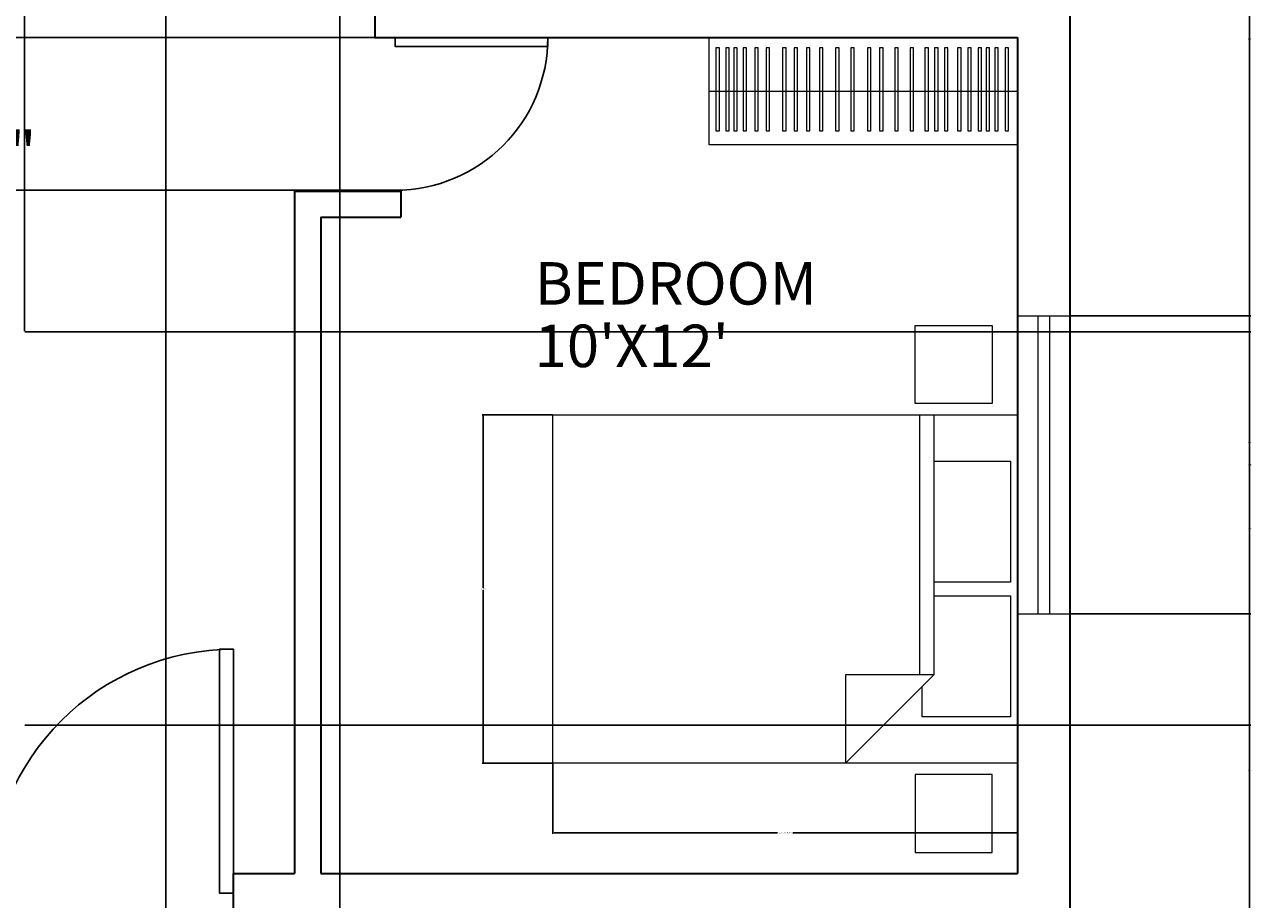
# Model space of a CAD drawing. Units: inches. Extents: x 25018 to 25490, y 41421 to 42101.
# Tile 4 of 5: x 25279 to 25490, y 41707 to 41858. Entities that reach past the tile are written whole.
import ezdxf

# ---------------------------------------------------------------- set-up
doc = ezdxf.new("R2010")
doc.units = ezdxf.units.IN
for name, color, linetype, lineweight in [('A-ANNO-DIMS', 2, 'Continuous', 18), ('A-AREA-IDEN', 7, 'Continuous', 18), ('A-DOOR', 3, 'Continuous', 25), ('A-FURN', 8, 'Continuous', 18), ('A-GLAZ', 4, 'Continuous', 18), ('A-WALL', 7, 'Continuous', 35)]:
    doc.layers.add(name, color=color, linetype=linetype, lineweight=lineweight)
doc.styles.get("Standard").update_dxf_attribs({"font": 'arial.ttf'})
doc.dimstyles.get("Standard").update_dxf_attribs({"dimtxt": 0.18, "dimasz": 0.18, "dimexe": 0.18, "dimexo": 0.0625, "dimgap": 0.09, "dimtad": 0, "dimtih": 1, "dimtoh": 1, "dimdec": 4, "dimzin": 0, "dimdsep": 46, "dimtxsty": 'Standard', "dimcen": 0.09, "dimadec": 0, "dimazin": 0, "dimtfac": 1, "dimtdec": 4, "dimtofl": 0, "dimtmove": 0, "dimatfit": 3, "dimfxl": 1, "dimtolj": 1, "dimtzin": 0, "dimarcsym": 0})

# ---------------------------------------------------------------- blocks, each defined once
blk = doc.blocks.new('*U2')
for p, q in [((0, 0), (0, -100)), ((750, 0), (750, -100))]:
    blk.add_line(p, q)
blk.add_lwpolyline([(0, 0), (0, 750), (43.75, 750), (43.75, 0)], close=True)
blk.add_arc((0, 0), 750, 0, 90)
blk = doc.blocks.new('Bed - Queen')
for p, q in [((0, -80.00003), (0, 0)), ((0, 0), (59.99999, 0)), ((59.99999, 0), (59.99999, -80.00003)), ((7.99999, -1.2), (28.79998, -1.2)), ((7.99999, -14.4), (7.99999, -1.2)), ((28.79998, -1.2), (28.79998, -14.4)), ((31.19999, -1.2), (51.99999, -1.2)), ((31.19999, -14.4), (31.19999, -1.2)), ((51.99999, -1.2), (51.99999, -16.4)), ((0, -14.4), (44.8, -14.4)), ((59.99999, -29.6), (44.8, -14.4)), ((44.8, -14.4), (44.8, -29.6)), ((44.8, -16.8), (0, -16.8)), ((51.99999, -16.4), (46.79936, -16.4)), ((44.8, -29.6), (59.99999, -29.6)), ((59.99999, -80.00003), (0, -80.00003))]:
    blk.add_line(p, q)
blk = doc.blocks.new('WARDROBE-SLATTED')
blk.add_line((0, 9.22), (53.1, 9.22))
for points in [[(0, 0), (53.1, 0), (53.1, 18.45), (0, 18.45)], [(1.16, 16.06), (1.76, 16.06), (1.76, 1.75), (1.16, 1.75)], [(2.87, 16.06), (3.47, 16.06), (3.47, 1.75), (2.87, 1.75)], [(4.23, 16.06), (4.83, 16.06), (4.83, 1.75), (4.23, 1.75)], [(5.83, 16.06), (6.43, 16.06), (6.43, 1.75), (5.83, 1.75)], [(7.85, 16.06), (8.45, 16.06), (8.45, 1.75), (7.85, 1.75)], [(9.82, 16.06), (10.42, 16.06), (10.42, 1.75), (9.82, 1.75)], [(12.64, 16.06), (13.24, 16.06), (13.24, 1.75), (12.64, 1.75)], [(14.63, 16.06), (15.23, 16.06), (15.23, 1.75), (14.63, 1.75)], [(16.74, 16.06), (17.34, 16.06), (17.34, 1.75), (16.74, 1.75)], [(18.99, 16.06), (19.59, 16.06), (19.59, 1.75), (18.99, 1.75)], [(21.77, 16.06), (22.37, 16.06), (22.37, 1.75), (21.77, 1.75)], [(24.4, 16.06), (25, 16.06), (25, 1.75), (24.4, 1.75)], [(27.25, 16.06), (27.85, 16.06), (27.85, 1.75), (27.25, 1.75)], [(29.36, 16.06), (29.96, 16.06), (29.96, 1.75), (29.36, 1.75)], [(31.98, 16.06), (32.58, 16.06), (32.58, 1.75), (31.98, 1.75)], [(34.61, 16.06), (35.21, 16.06), (35.21, 1.75), (34.61, 1.75)], [(37.17, 16.06), (37.77, 16.06), (37.77, 1.75), (37.17, 1.75)], [(38.82, 16.06), (39.42, 16.06), (39.42, 1.75), (38.82, 1.75)], [(40.51, 16.06), (41.11, 16.06), (41.11, 1.75), (40.51, 1.75)], [(42.78, 16.06), (43.38, 16.06), (43.38, 1.75), (42.78, 1.75)], [(44.55, 16.06), (45.15, 16.06), (45.15, 1.75), (44.55, 1.75)], [(46.32, 16.06), (46.92, 16.06), (46.92, 1.75), (46.32, 1.75)], [(47.7, 16.06), (48.3, 16.06), (48.3, 1.75), (47.7, 1.75)], [(49.2, 16.06), (49.8, 16.06), (49.8, 1.75), (49.2, 1.75)], [(50.97, 16.06), (51.57, 16.06), (51.57, 1.75), (50.97, 1.75)]]:
    blk.add_lwpolyline(points, close=True)
blk = doc.blocks.new('TABLE-BEDSIDE')
blk.add_lwpolyline([(0, 13.4), (13.26, 13.4), (13.26, 0), (0, 0)], close=True)
blk = doc.blocks.new('*D18')
at = {"layer": 'A-ANNO-DIMS', "color": 0, "lineweight": -2, "transparency": 16777216}
for p, q in [((25369.65, 41730.48), (25369.65, 41718.36)), ((25449.65, 41730.48), (25449.65, 41718.36)), ((25369.83, 41718.54), (25408.35, 41718.54)), ((25449.47, 41718.54), (25410.96, 41718.54))]:
    blk.add_line(p, q, dxfattribs=at)
at = {"layer": 'A-ANNO-DIMS', "color": 0, "transparency": 16777216}
for points in [[(25369.83, 41718.57), (25369.83, 41718.51), (25369.65, 41718.54)], [(25449.47, 41718.57), (25449.47, 41718.51), (25449.65, 41718.54)]]:
    blk.add_solid(points, dxfattribs=at)
at = {"layer": 'Defpoints', "color": 0, "transparency": 16777216}
for p in [(25369.65, 41730.54), (25449.65, 41730.54), (25449.65, 41718.54)]:
    blk.add_point(p, dxfattribs=at)
at = {"layer": 'A-ANNO-DIMS', "color": 0, "transparency": 16777216, "insert": (25409.65, 41718.54), "char_height": 0.18, "attachment_point": 5}
blk.add_mtext('\\A1;QUEEN BED 80 TYP.', dxfattribs=at)
blk = doc.blocks.new('*D19')
at = {"layer": 'A-ANNO-DIMS', "color": 0, "lineweight": -2, "transparency": 16777216}
for p, q in [((25369.59, 41790.54), (25357.47, 41790.54)), ((25357.65, 41790.36), (25357.65, 41760.72)), ((25357.65, 41730.72), (25357.65, 41760.36)), ((25369.59, 41730.54), (25357.47, 41730.54))]:
    blk.add_line(p, q, dxfattribs=at)
at = {"layer": 'A-ANNO-DIMS', "color": 0, "transparency": 16777216}
for points in [[(25357.62, 41790.36), (25357.68, 41790.36), (25357.65, 41790.54)], [(25357.62, 41730.72), (25357.68, 41730.72), (25357.65, 41730.54)]]:
    blk.add_solid(points, dxfattribs=at)
at = {"layer": 'Defpoints', "color": 0, "transparency": 16777216}
for p in [(25369.65, 41790.54), (25357.65, 41730.54), (25369.65, 41730.54)]:
    blk.add_point(p, dxfattribs=at)
at = {"layer": 'A-ANNO-DIMS', "color": 0, "transparency": 16777216, "insert": (25357.65, 41760.54), "char_height": 0.18, "attachment_point": 5}
blk.add_mtext('\\A1;60 TYP.', dxfattribs=at)
blk = doc.blocks.new('*D39')
at = {"layer": 'A-ANNO-DIMS', "color": 0, "lineweight": -2, "transparency": 16777216}
for p, q in [((25458.72, 42070.05), (25489.83, 42070.05)), ((25489.65, 42069.87), (25489.65, 41785.98)), ((25489.65, 41501.73), (25489.65, 41785.62)), ((25458.72, 41501.55), (25489.83, 41501.55))]:
    blk.add_line(p, q, dxfattribs=at)
at = {"layer": 'A-ANNO-DIMS', "color": 0, "transparency": 16777216}
for points in [[(25489.62, 42069.87), (25489.68, 42069.87), (25489.65, 42070.05)], [(25489.62, 41501.73), (25489.68, 41501.73), (25489.65, 41501.55)]]:
    blk.add_solid(points, dxfattribs=at)
at = {"layer": 'Defpoints', "color": 0, "transparency": 16777216}
for p in [(25458.65, 42070.05), (25489.65, 42070.05), (25458.65, 41501.55)]:
    blk.add_point(p, dxfattribs=at)
at = {"layer": 'A-ANNO-DIMS', "color": 0, "transparency": 16777216, "insert": (25489.65, 41785.8), "char_height": 0.18, "attachment_point": 5}
blk.add_mtext('\\A1;568.5', dxfattribs=at)
blk = doc.blocks.new('*D54')
at = {"layer": 'A-ANNO-DIMS', "color": 0, "lineweight": -2, "transparency": 16777216}
for p, q in [((25458.72, 41756.26), (25489.83, 41756.26)), ((25489.65, 41756.08), (25489.65, 41729.59)), ((25489.65, 41702.73), (25489.65, 41729.22)), ((25458.72, 41702.55), (25489.83, 41702.55))]:
    blk.add_line(p, q, dxfattribs=at)
at = {"layer": 'A-ANNO-DIMS', "color": 0, "transparency": 16777216}
for points in [[(25489.62, 41756.08), (25489.68, 41756.08), (25489.65, 41756.26)], [(25489.62, 41702.73), (25489.68, 41702.73), (25489.65, 41702.55)]]:
    blk.add_solid(points, dxfattribs=at)
at = {"layer": 'Defpoints', "color": 0, "transparency": 16777216}
for p in [(25458.65, 41756.26), (25489.65, 41756.26), (25458.65, 41702.55)]:
    blk.add_point(p, dxfattribs=at)
at = {"layer": 'A-ANNO-DIMS', "color": 0, "transparency": 16777216, "insert": (25489.65, 41729.4), "char_height": 0.18, "attachment_point": 5}
blk.add_mtext('\\A1;53.71', dxfattribs=at)
blk = doc.blocks.new('*D55')
at = {"layer": 'A-ANNO-DIMS', "color": 0, "lineweight": -2, "transparency": 16777216}
for p, q in [((25458.72, 41807.63), (25489.83, 41807.63)), ((25489.65, 41807.45), (25489.65, 41782.13)), ((25489.65, 41756.44), (25489.65, 41781.76)), ((25458.72, 41756.26), (25489.83, 41756.26))]:
    blk.add_line(p, q, dxfattribs=at)
at = {"layer": 'A-ANNO-DIMS', "color": 0, "transparency": 16777216}
for points in [[(25489.62, 41807.45), (25489.68, 41807.45), (25489.65, 41807.63)], [(25489.62, 41756.44), (25489.68, 41756.44), (25489.65, 41756.26)]]:
    blk.add_solid(points, dxfattribs=at)
at = {"layer": 'Defpoints', "color": 0, "transparency": 16777216}
for p in [(25458.65, 41807.63), (25489.65, 41807.63), (25458.65, 41756.26)]:
    blk.add_point(p, dxfattribs=at)
at = {"layer": 'A-ANNO-DIMS', "color": 0, "transparency": 16777216, "insert": (25489.65, 41781.95), "char_height": 0.18, "attachment_point": 5}
blk.add_mtext('\\A1;51.38', dxfattribs=at)
blk = doc.blocks.new('*D56')
at = {"layer": 'A-ANNO-DIMS', "color": 0, "lineweight": -2, "transparency": 16777216}
for p, q in [((25458.72, 41903), (25489.83, 41903)), ((25489.65, 41902.82), (25489.65, 41855.5)), ((25489.65, 41807.81), (25489.65, 41855.13)), ((25458.72, 41807.63), (25489.83, 41807.63))]:
    blk.add_line(p, q, dxfattribs=at)
at = {"layer": 'A-ANNO-DIMS', "color": 0, "transparency": 16777216}
for points in [[(25489.62, 41902.82), (25489.68, 41902.82), (25489.65, 41903)], [(25489.62, 41807.81), (25489.68, 41807.81), (25489.65, 41807.63)]]:
    blk.add_solid(points, dxfattribs=at)
at = {"layer": 'Defpoints', "color": 0, "transparency": 16777216}
for p in [(25458.65, 41903), (25489.65, 41903), (25458.65, 41807.63)]:
    blk.add_point(p, dxfattribs=at)
at = {"layer": 'A-ANNO-DIMS', "color": 0, "transparency": 16777216, "insert": (25489.65, 41855.31), "char_height": 0.18, "attachment_point": 5}
blk.add_mtext('\\A1;95.36', dxfattribs=at)
blk = doc.blocks.new('*D70')
at = {"layer": 'A-ANNO-DIMS', "color": 0, "lineweight": -2, "transparency": 16777216}
for p, q in [((25250.45, 41903.49), (25250.45, 41420.7)), ((25302.95, 41903.49), (25302.95, 41420.7)), ((25250.63, 41420.88), (25276.38, 41420.88)), ((25302.77, 41420.88), (25277.03, 41420.88))]:
    blk.add_line(p, q, dxfattribs=at)
at = {"layer": 'A-ANNO-DIMS', "color": 0, "transparency": 16777216}
for points in [[(25250.63, 41420.91), (25250.63, 41420.85), (25250.45, 41420.88)], [(25302.77, 41420.91), (25302.77, 41420.85), (25302.95, 41420.88)]]:
    blk.add_solid(points, dxfattribs=at)
at = {"layer": 'Defpoints', "color": 0, "transparency": 16777216}
for p in [(25250.45, 41903.55), (25302.95, 41903.55), (25302.95, 41420.88)]:
    blk.add_point(p, dxfattribs=at)
at = {"layer": 'A-ANNO-DIMS', "color": 0, "transparency": 16777216, "insert": (25276.7, 41420.88), "char_height": 0.18, "attachment_point": 5}
blk.add_mtext('\\A1;52.5', dxfattribs=at)
blk = doc.blocks.new('*D71')
at = {"layer": 'A-ANNO-DIMS', "color": 0, "lineweight": -2, "transparency": 16777216}
for p, q in [((25302.95, 41903.49), (25302.95, 41420.7)), ((25332.95, 41903.49), (25332.95, 41420.7)), ((25303.13, 41420.88), (25317.73, 41420.88)), ((25332.77, 41420.88), (25318.17, 41420.88))]:
    blk.add_line(p, q, dxfattribs=at)
at = {"layer": 'A-ANNO-DIMS', "color": 0, "transparency": 16777216}
for points in [[(25303.13, 41420.91), (25303.13, 41420.85), (25302.95, 41420.88)], [(25332.77, 41420.91), (25332.77, 41420.85), (25332.95, 41420.88)]]:
    blk.add_solid(points, dxfattribs=at)
at = {"layer": 'Defpoints', "color": 0, "transparency": 16777216}
for p in [(25302.95, 41903.55), (25332.95, 41903.55), (25332.95, 41420.88)]:
    blk.add_point(p, dxfattribs=at)
at = {"layer": 'A-ANNO-DIMS', "color": 0, "transparency": 16777216, "insert": (25317.95, 41420.88), "char_height": 0.18, "attachment_point": 5}
blk.add_mtext('\\A1;30', dxfattribs=at)
blk = doc.blocks.new('*D73')
at = {"layer": 'A-ANNO-DIMS', "color": 0, "lineweight": -2, "transparency": 16777216}
for p, q in [((25338.89, 41855.55), (25018.58, 41855.55)), ((25018.76, 41855.37), (25018.76, 41842.58)), ((25018.76, 41829.43), (25018.76, 41842.22)), ((25338.89, 41829.25), (25018.58, 41829.25))]:
    blk.add_line(p, q, dxfattribs=at)
at = {"layer": 'A-ANNO-DIMS', "color": 0, "transparency": 16777216}
for points in [[(25018.73, 41855.37), (25018.79, 41855.37), (25018.76, 41855.55)], [(25018.73, 41829.43), (25018.79, 41829.43), (25018.76, 41829.25)]]:
    blk.add_solid(points, dxfattribs=at)
at = {"layer": 'Defpoints', "color": 0, "transparency": 16777216}
for p in [(25018.76, 41855.55), (25338.95, 41855.55), (25338.95, 41829.25)]:
    blk.add_point(p, dxfattribs=at)
at = {"layer": 'A-ANNO-DIMS', "color": 0, "transparency": 16777216, "insert": (25018.76, 41842.4), "char_height": 0.18, "attachment_point": 5}
blk.add_mtext('\\A1;26.3', dxfattribs=at)
blk = doc.blocks.new('*D75')
at = {"layer": 'A-ANNO-DIMS', "color": 0, "lineweight": -2, "transparency": 16777216}
for p, q in [((25201.64, 41804.94), (25201.64, 42101.23)), ((25201.82, 42101.05), (25239.92, 42101.05)), ((25278.45, 42101.05), (25240.36, 42101.05)), ((25278.63, 41804.94), (25278.63, 42101.23))]:
    blk.add_line(p, q, dxfattribs=at)
at = {"layer": 'A-ANNO-DIMS', "color": 0, "transparency": 16777216}
for points in [[(25201.82, 42101.08), (25201.82, 42101.02), (25201.64, 42101.05)], [(25278.45, 42101.08), (25278.45, 42101.02), (25278.63, 42101.05)]]:
    blk.add_solid(points, dxfattribs=at)
at = {"layer": 'Defpoints', "color": 0, "transparency": 16777216}
for p in [(25278.63, 42101.05), (25201.64, 41804.88), (25278.63, 41804.88)]:
    blk.add_point(p, dxfattribs=at)
at = {"layer": 'A-ANNO-DIMS', "color": 0, "transparency": 16777216, "insert": (25240.14, 42101.05), "char_height": 0.18, "attachment_point": 5}
blk.add_mtext('\\A1;77', dxfattribs=at)
blk = doc.blocks.new('*D76')
at = {"layer": 'A-ANNO-DIMS', "color": 0, "lineweight": -2, "transparency": 16777216}
for p, q in [((25278.7, 41804.88), (25489.83, 41804.88)), ((25489.65, 41804.7), (25489.65, 41771.17)), ((25489.65, 41737.28), (25489.65, 41770.81)), ((25278.7, 41737.1), (25489.83, 41737.1))]:
    blk.add_line(p, q, dxfattribs=at)
at = {"layer": 'A-ANNO-DIMS', "color": 0, "transparency": 16777216}
for points in [[(25489.62, 41804.7), (25489.68, 41804.7), (25489.65, 41804.88)], [(25489.62, 41737.28), (25489.68, 41737.28), (25489.65, 41737.1)]]:
    blk.add_solid(points, dxfattribs=at)
at = {"layer": 'Defpoints', "color": 0, "transparency": 16777216}
for p in [(25278.63, 41804.88), (25278.63, 41737.1), (25489.65, 41737.1)]:
    blk.add_point(p, dxfattribs=at)
at = {"layer": 'A-ANNO-DIMS', "color": 0, "transparency": 16777216, "insert": (25489.65, 41770.99), "char_height": 0.18, "attachment_point": 5}
blk.add_mtext('\\A1;67.78', dxfattribs=at)

msp = doc.modelspace()

# ---------------------------------------------------------------- linework, layer by layer
at = {"layer": 'A-GLAZ'}
for p, q in [((25449.6526, 41807.6331), (25458.6526, 41807.6331)), ((25453.1526, 41807.6331), (25453.1526, 41756.2579)), ((25455.1526, 41807.6331), (25455.1526, 41756.2579)), ((25449.6526, 41756.2579), (25458.6526, 41756.2579))]:
    msp.add_line(p, q, dxfattribs=at)
at = {"layer": 'A-WALL'}
for p, q in [((25458.6526, 42070.0498), (25458.6526, 41501.5498)), ((25338.9527, 41860.0498), (25338.9527, 41855.5498)), ((25338.9527, 41855.5498), (25449.6526, 41855.5498)), ((25449.6526, 41855.5498), (25449.6526, 41711.5498)), ((25325.1526, 41829.1098), (25325.1526, 41711.5498)), ((25325.1526, 41829.1098), (25343.4527, 41829.1098)), ((25343.4527, 41829.1098), (25343.4527, 41824.6098)), ((25329.6526, 41824.6098), (25329.6526, 41711.5498)), ((25329.6526, 41824.6098), (25343.4527, 41824.6098)), ((25314.6526, 41711.5498), (25325.1526, 41711.5498)), ((25314.6526, 41702.5498), (25314.6526, 41711.5498)), ((25329.6526, 41711.5498), (25449.6526, 41711.5498))]:
    msp.add_line(p, q, dxfattribs=at)

# ---------------------------------------------------------------- block references
at = {"layer": 'A-DOOR', "xscale": 0.0350684013995968, "yscale": 0.0350684013995968, "zscale": 0.0350684013995968, "rotation": 270}
msp.add_blockref('*U2', (25342.4595, 41855.5498), dxfattribs=at)
at = {"layer": 'A-DOOR', "xscale": -0.0560000000000015, "yscale": 0.0560000000000015, "zscale": 0.0560000000000015}
msp.add_blockref('*U2', (25314.6526, 41708.1498), dxfattribs=at)
at = {"layer": 'A-FURN', "extrusion": (0, 0, -1), "zscale": -1, "rotation": 180}
for name, p in [('WARDROBE-SLATTED', (-25396.553, 41855.5497)), ('TABLE-BEDSIDE', (-25432.0295, 41728.563))]:
    msp.add_blockref(name, p, dxfattribs=at)
at = {"layer": 'A-FURN'}
msp.add_blockref('TABLE-BEDSIDE', (25432.0295, 41792.5192), dxfattribs=at)
at = {"layer": 'A-FURN', "rotation": 270}
msp.add_blockref('Bed - Queen', (25449.6526, 41790.5411), dxfattribs=at)

# ---------------------------------------------------------------- texts
at = {"layer": 'A-AREA-IDEN'}
for s, p in [('15\'6"X8\'0"', (25232.2006, 41832.0193)), ('BEDROOM', (25366.4994, 41809.5363)), ("10'X12'", (25366.5071, 41798.7771))]:
    msp.add_text(s, height=7.32047, dxfattribs=at).set_placement(p)

# ---------------------------------------------------------------- dimensions: what is measured, and where the dimension line sits
at = {"layer": 'A-ANNO-DIMS'}
for base, p1, p2, override, picture, middle in [((25278.6341, 42101.0498), (25201.6418, 41804.8791), (25278.6341, 41804.8791), {"dimdec": 0, "dimlfac": 1, "dimrnd": 0, "dimzin": 0, "dimdsep": 46, "dimlunit": 2}, '*D75', (25240.138, 42101.0498)), ((25302.9527, 41420.8835), (25250.4527, 41903.5498), (25302.9527, 41903.5498), {"dimdec": 1, "dimlfac": 1, "dimrnd": 0, "dimzin": 0, "dimdsep": 46, "dimlunit": 2}, '*D70', (25276.7027, 41420.8835)), ((25332.9527, 41420.8835), (25302.9527, 41903.5498), (25332.9527, 41903.5498), {"dimdec": 0, "dimlfac": 1, "dimrnd": 0, "dimzin": 0, "dimdsep": 46, "dimlunit": 2}, '*D71', (25317.9527, 41420.8835))]:
    dim = msp.add_linear_dim(base=base, p1=p1, p2=p2, dimstyle='Standard', override=override, dxfattribs=at)
    dim.commit()
    dim.dimension.update_dxf_attribs({"geometry": picture, "text_midpoint": middle})
for base, p1, p2, override, picture, middle in [((25489.6526, 42070.0498), (25458.6526, 41501.5498), (25458.6526, 42070.0498), {"dimdec": 1, "dimlfac": 1, "dimrnd": 0, "dimzin": 0, "dimdsep": 46, "dimlunit": 2}, '*D39', (25489.6526, 41785.7998)), ((25489.6526, 41902.9968), (25458.6526, 41807.6331), (25458.6526, 41902.9968), {"dimdec": 2, "dimlfac": 1, "dimrnd": 0, "dimzin": 0, "dimdsep": 46, "dimlunit": 2}, '*D56', (25489.6526, 41855.315)), ((25018.7568, 41855.5498), (25338.9527, 41829.2485), (25338.9527, 41855.5498), {"dimdec": 1, "dimlfac": 1, "dimrnd": 0, "dimzin": 0, "dimdsep": 46, "dimlunit": 2}, '*D73', (25018.7568, 41842.3992)), ((25489.6526, 41807.6331), (25458.6526, 41756.2579), (25458.6526, 41807.6331), {"dimdec": 2, "dimlfac": 1, "dimrnd": 0, "dimzin": 0, "dimdsep": 46, "dimlunit": 2}, '*D55', (25489.6526, 41781.9455)), ((25489.6526, 41737.1033), (25278.6341, 41804.8791), (25278.6341, 41737.1033), {"dimdec": 2, "dimlfac": 1, "dimrnd": 0, "dimzin": 0, "dimdsep": 46, "dimlunit": 2}, '*D76', (25489.6526, 41770.9912)), ((25489.6526, 41756.2579), (25458.6526, 41702.5498), (25458.6526, 41756.2579), {"dimdec": 2, "dimlfac": 1, "dimrnd": 0, "dimzin": 0, "dimdsep": 46, "dimlunit": 2}, '*D54', (25489.6526, 41729.4039))]:
    dim = msp.add_linear_dim(base=base, p1=p1, p2=p2, angle=90, dimstyle='Standard', override=override, dxfattribs=at)
    dim.commit()
    dim.dimension.update_dxf_attribs({"geometry": picture, "text_midpoint": middle})
dim = msp.add_linear_dim(base=(25357.6526, 41730.5411), p1=(25369.6526, 41790.5411), p2=(25369.6526, 41730.5411), angle=270, text='<> TYP.', dimstyle='Standard', override={"dimdec": 0, "dimlfac": 1, "dimrnd": 0, "dimzin": 0, "dimdsep": 46, "dimlunit": 2}, dxfattribs=at)
dim.commit()
dim.dimension.update_dxf_attribs({"geometry": '*D19', "text_midpoint": (25357.6526, 41760.5411)})
dim = msp.add_linear_dim(base=(25449.6526, 41718.5411), p1=(25369.6526, 41730.5411), p2=(25449.6526, 41730.5411), text='QUEEN BED <> TYP.', dimstyle='Standard', override={"dimdec": 0, "dimlfac": 1, "dimrnd": 0, "dimzin": 0, "dimdsep": 46, "dimlunit": 2}, dxfattribs=at)
dim.commit()
dim.dimension.update_dxf_attribs({"geometry": '*D18', "text_midpoint": (25409.6526, 41718.5411)})

doc.saveas('drawing.dxf')
